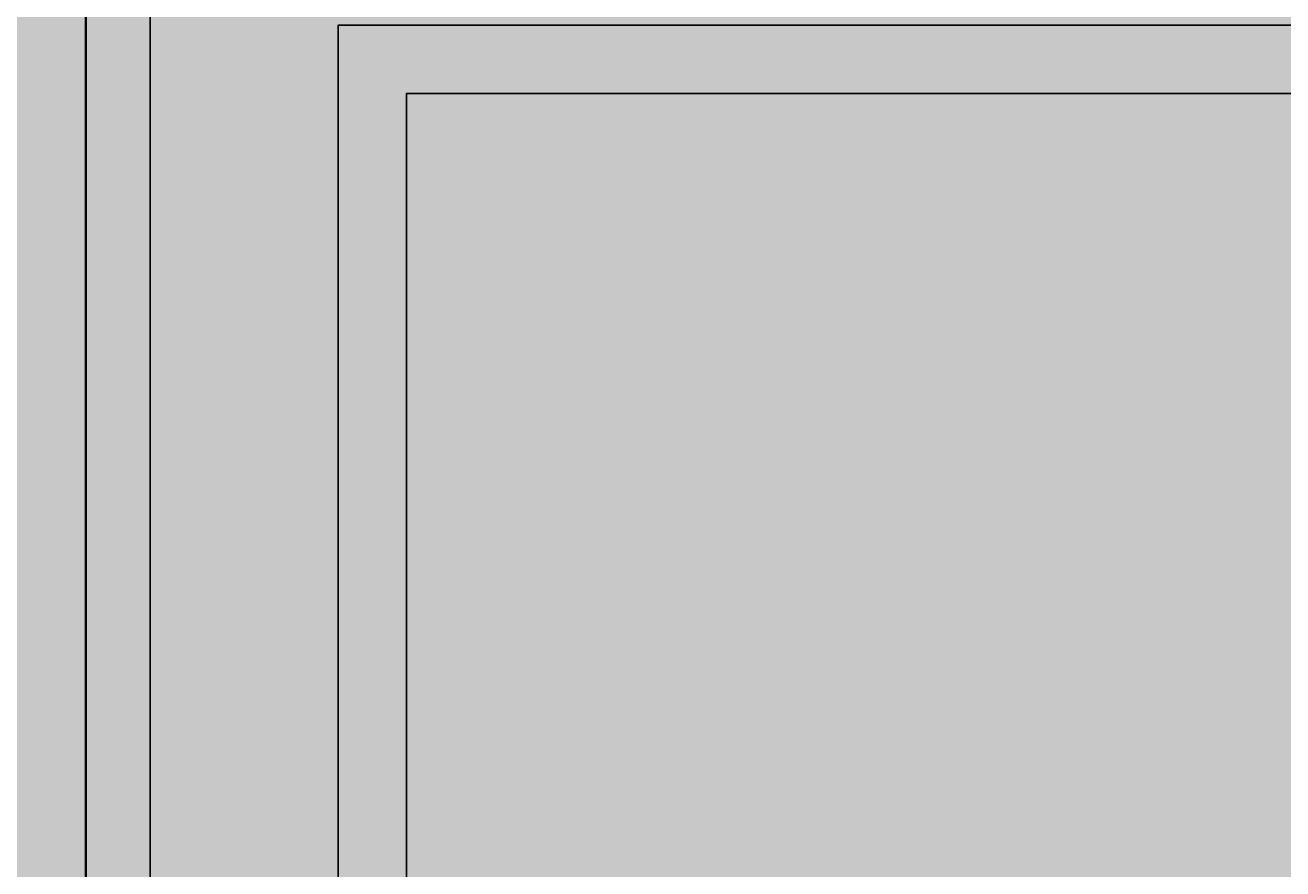
# Model space of a CAD drawing. Units: feet. Extents: x 2695 to 2912, y 795 to 1139.
# Tile 54 of 83: x 2769 to 2806, y 996 to 1021. Entities that reach past the tile are written whole.
import ezdxf

# ---------------------------------------------------------------- set-up
doc = ezdxf.new("R2010")
doc.units = ezdxf.units.FT
for name, color, linetype, lineweight in [('A-ANNO-DIMS', 2, 'Continuous', 18), ('A-ELEV', 7, 'Continuous', 35), ('A-ELEV-PATT', 252, 'Continuous', 13), ('A-GLAZ', 4, 'Continuous', 25), ('A-GLAZ-PATT', 254, 'Continuous', 13)]:
    doc.layers.add(name, color=color, linetype=linetype, lineweight=lineweight)
doc.styles.get("Standard").update_dxf_attribs({"font": 'arial.ttf'})
doc.dimstyles.get("Standard").update_dxf_attribs({"dimtxt": 0.18, "dimasz": 0.18, "dimexe": 0.18, "dimexo": 0.0625, "dimgap": 0.09, "dimtad": 0, "dimtih": 1, "dimtoh": 1, "dimdec": 1, "dimzin": 0, "dimdsep": 46, "dimlunit": 3, "dimtxsty": 'Standard', "dimcen": 0.09, "dimadec": 0, "dimazin": 0, "dimtfac": 1, "dimtdec": 1, "dimtofl": 0, "dimtmove": 0, "dimatfit": 3, "dimfxl": 1, "dimtolj": 1, "dimtzin": 0, "dimarcsym": 0})

# ---------------------------------------------------------------- blocks, each defined once
blk = doc.blocks.new('*D48')
at = {"layer": 'A-ANNO-DIMS', "color": 0, "lineweight": -2, "transparency": 16777216}
for p, q in [((2770.636, 972.03), (2770.636, 1138.886)), ((2770.816, 1138.706), (2771.263, 1138.706)), ((2772.342, 1138.706), (2771.894, 1138.706)), ((2772.522, 972.03), (2772.522, 1138.886))]:
    blk.add_line(p, q, dxfattribs=at)
at = {"layer": 'A-ANNO-DIMS', "color": 0, "transparency": 16777216}
for points in [[(2770.816, 1138.736), (2770.816, 1138.676), (2770.636, 1138.706)], [(2772.342, 1138.736), (2772.342, 1138.676), (2772.522, 1138.706)]]:
    blk.add_solid(points, dxfattribs=at)
at = {"layer": 'Defpoints', "color": 0, "transparency": 16777216}
for p in [(2772.522, 1138.706), (2770.636, 971.967), (2772.522, 971.967)]:
    blk.add_point(p, dxfattribs=at)
at = {"layer": 'A-ANNO-DIMS', "color": 0, "transparency": 16777216, "insert": (2771.579, 1138.706), "char_height": 0.18, "attachment_point": 5}
blk.add_mtext('\\A1;1.89', dxfattribs=at)
blk = doc.blocks.new('*D49')
at = {"layer": 'A-ANNO-DIMS', "color": 0, "lineweight": -2, "transparency": 16777216}
for p, q in [((2772.522, 972.03), (2772.522, 1138.886)), ((2772.702, 1138.706), (2790.888, 1138.706)), ((2809.861, 1138.706), (2791.674, 1138.706)), ((2810.041, 972.03), (2810.041, 1138.886))]:
    blk.add_line(p, q, dxfattribs=at)
at = {"layer": 'A-ANNO-DIMS', "color": 0, "transparency": 16777216}
for points in [[(2772.702, 1138.736), (2772.702, 1138.676), (2772.522, 1138.706)], [(2809.861, 1138.736), (2809.861, 1138.676), (2810.041, 1138.706)]]:
    blk.add_solid(points, dxfattribs=at)
at = {"layer": 'Defpoints', "color": 0, "transparency": 16777216}
for p in [(2810.041, 1138.706), (2772.522, 971.967), (2810.041, 971.967)]:
    blk.add_point(p, dxfattribs=at)
at = {"layer": 'A-ANNO-DIMS', "color": 0, "transparency": 16777216, "insert": (2791.281, 1138.706), "char_height": 0.18, "attachment_point": 5}
blk.add_mtext('\\A1;37.52', dxfattribs=at)

msp = doc.modelspace()

# ---------------------------------------------------------------- hatches: boundary and pattern name
at = {"layer": 'A-ELEV-PATT'}
h = msp.add_hatch(color=256, dxfattribs=at)
h.set_gradient(color1=(147, 149, 152), color2=(147, 149, 152), tint=1)
h.paths.add_polyline_path([(2770.6361, 1118.4096), (2710.6361, 1118.4096), (2710.6361, 1062.9306), (2770.6361, 1062.9306)])
h.paths.add_polyline_path([(2890.6361, 1103.3378), (2770.6361, 1103.3378), (2770.6361, 1062.9306), (2890.6361, 1062.9306)])
h.paths.add_polyline_path([(2730.7081, 1048.1052), (2755.1125, 1048.1052), (2755.1125, 936.9306), (2770.6361, 936.9306), (2770.6361, 1050.3105), (2715.8852, 1050.3105), (2715.8852, 936.9306), (2730.7081, 936.9306)])
h.paths.add_polyline_path([(2890.6361, 1050.3105), (2770.6361, 1050.3105), (2770.6361, 971.9673), (2778.0341, 971.9673), (2778.0341, 1020.8235), (2843.575, 1020.8235), (2843.575, 971.9673), (2890.6361, 971.9673)])
h.paths.add_polyline_path([(2888.1882, 970.7156), (2843.575, 970.7156), (2843.575, 964.8267), (2888.1882, 964.8267)])
h.paths.add_polyline_path([(2888.1882, 964.1328), (2843.575, 964.1328), (2843.575, 956.614), (2888.1882, 956.614)])
h.paths.add_polyline_path([(2888.1882, 955.9202), (2843.575, 955.9202), (2843.575, 949.2892), (2888.1882, 949.2892)])
h.paths.add_polyline_path([(2888.1882, 948.5954), (2843.575, 948.5954), (2843.575, 941.3507), (2888.1882, 941.3507)])
h.paths.add_polyline_path([(2888.1882, 940.6569), (2843.575, 940.6569), (2843.575, 936.9306), (2888.1882, 936.9306)])
h.paths.add_polyline_path([(2890.6361, 970.7156), (2888.9368, 970.7156), (2888.9368, 964.8267), (2890.6361, 964.8267)])
h.paths.add_polyline_path([(2890.6361, 964.1328), (2888.9368, 964.1328), (2888.9368, 956.614), (2890.6361, 956.614)])
h.paths.add_polyline_path([(2890.6361, 955.9202), (2888.9368, 955.9202), (2888.9368, 949.2892), (2890.6361, 949.2892)])
h.paths.add_polyline_path([(2890.6361, 940.6569), (2888.9368, 940.6569), (2888.9368, 936.9306), (2890.6361, 936.9306)])
h.paths.add_polyline_path([(2890.6361, 948.5954), (2888.9368, 948.5954), (2888.9368, 941.3507), (2890.6361, 941.3507)])
h.paths.add_polyline_path([(2772.5216, 970.7156), (2770.6361, 970.7156), (2770.6361, 964.8267), (2772.5216, 964.8267)])
h.paths.add_polyline_path([(2772.5216, 964.1328), (2770.6361, 964.1328), (2770.6361, 956.614), (2772.5216, 956.614)])
h.paths.add_polyline_path([(2772.5216, 955.9202), (2770.6361, 955.9202), (2770.6361, 949.2892), (2772.5216, 949.2892)])
h.paths.add_polyline_path([(2772.5216, 948.5954), (2770.6361, 948.5954), (2770.6361, 941.3507), (2772.5216, 941.3507)])
h.paths.add_polyline_path([(2772.5216, 940.6569), (2770.6361, 940.6569), (2770.6361, 936.9306), (2772.5216, 936.9306)])
h.paths.add_polyline_path([(2778.0341, 940.6569), (2773.2702, 940.6569), (2773.2702, 936.9306), (2778.0341, 936.9306)])
h.paths.add_polyline_path([(2778.0341, 970.7156), (2773.2702, 970.7156), (2773.2702, 964.8267), (2778.0341, 964.8267)])
h.paths.add_polyline_path([(2778.0341, 964.1328), (2773.2702, 964.1328), (2773.2702, 956.614), (2778.0341, 956.614)])
h.paths.add_polyline_path([(2778.0341, 955.9202), (2773.2702, 955.9202), (2773.2702, 949.2892), (2778.0341, 949.2892)])
h.paths.add_polyline_path([(2778.0341, 948.5954), (2773.2702, 948.5954), (2773.2702, 941.3507), (2778.0341, 941.3507)])
h.paths.add_polyline_path([(2810.0407, 940.6569), (2780.0341, 940.6569), (2780.0341, 936.9306), (2810.0407, 936.9306)])
h.paths.add_polyline_path([(2890.6361, 924.3105), (2770.6361, 924.3105), (2770.6361, 810.9306), (2773.5029, 810.9306), (2773.5029, 905.5143), (2805.9398, 905.5143), (2838.3767, 905.5143), (2838.3767, 810.9306), (2890.6361, 810.9306)])
h = msp.add_hatch(color=256, dxfattribs=at)
h.set_gradient(color2=(0, 0, 0), tint=1)
h.paths.add_polyline_path([(2772.5216, 971.9673), (2770.6361, 971.9673), (2770.6361, 970.7156), (2772.5216, 970.7156)])
h.paths.add_polyline_path([(2773.2702, 971.9673), (2772.5216, 971.9673), (2772.5216, 970.7156), (2773.2702, 970.7156)])
h.paths.add_polyline_path([(2778.0341, 971.9673), (2773.2702, 971.9673), (2773.2702, 970.7156), (2778.0341, 970.7156)])
h.paths.add_polyline_path([(2780.0341, 971.9673), (2778.0341, 971.9673), (2778.0341, 970.7156), (2780.0341, 970.7156)])
h.paths.add_polyline_path([(2841.575, 971.9673), (2780.0341, 971.9673), (2780.0341, 970.7156), (2841.575, 970.7156)])
h.paths.add_polyline_path([(2843.575, 971.9673), (2841.575, 971.9673), (2841.575, 970.7156), (2843.575, 970.7156)])
h.paths.add_polyline_path([(2888.1882, 971.9673), (2843.575, 971.9673), (2843.575, 970.7156), (2888.1882, 970.7156)])
h.paths.add_polyline_path([(2888.9368, 971.9673), (2888.1882, 971.9673), (2888.1882, 970.7156), (2888.9368, 970.7156)], flags=17)
h.paths.add_polyline_path([(2890.6361, 971.9673), (2888.9368, 971.9673), (2888.9368, 970.7156), (2890.6361, 970.7156)])
h.paths.add_polyline_path([(2888.9368, 971.9673), (2888.1882, 971.9673), (2888.1882, 964.8267), (2888.9368, 964.8267)])
h.paths.add_polyline_path([(2888.9368, 964.8267), (2888.1882, 964.8267), (2888.1882, 964.1328), (2888.9368, 964.1328)])
h.paths.add_polyline_path([(2890.6361, 964.8267), (2888.9368, 964.8267), (2888.9368, 964.1328), (2890.6361, 964.1328)])
h.paths.add_polyline_path([(2888.1882, 964.8267), (2770.6361, 964.8267), (2770.6361, 964.1328), (2888.1882, 964.1328)])
h.paths.add_polyline_path([(2888.9368, 964.1328), (2888.1882, 964.1328), (2888.1882, 936.9306), (2888.9368, 936.9306)])
h.paths.add_polyline_path([(2890.6361, 956.614), (2888.9368, 956.614), (2888.9368, 955.9202), (2890.6361, 955.9202)])
h.paths.add_polyline_path([(2888.1882, 956.614), (2770.6361, 956.614), (2770.6361, 955.9202), (2888.1882, 955.9202)])
h.paths.add_polyline_path([(2890.6361, 949.2892), (2888.9368, 949.2892), (2888.9368, 948.5954), (2890.6361, 948.5954)])
h.paths.add_polyline_path([(2888.1882, 949.2892), (2770.6361, 949.2892), (2770.6361, 948.5954), (2888.1882, 948.5954)])
h.paths.add_polyline_path([(2890.6361, 941.3507), (2888.9368, 941.3507), (2888.9368, 940.6569), (2890.6361, 940.6569)])
h.paths.add_polyline_path([(2888.1882, 941.3507), (2770.6361, 941.3507), (2770.6361, 940.6569), (2888.1882, 940.6569)])
h.paths.add_polyline_path([(2773.2702, 970.7156), (2772.5216, 970.7156), (2772.5216, 964.8267), (2773.2702, 964.8267)])
h.paths.add_polyline_path([(2773.2702, 964.1328), (2772.5216, 964.1328), (2772.5216, 956.614), (2773.2702, 956.614)])
h.paths.add_polyline_path([(2773.2702, 955.9202), (2772.5216, 955.9202), (2772.5216, 936.9306), (2773.2702, 936.9306)])
h.paths.add_polyline_path([(2810.7893, 970.7156), (2810.0407, 970.7156), (2810.0407, 964.8267), (2810.7893, 964.8267)], flags=17)
h.paths.add_polyline_path([(2810.7893, 964.1328), (2810.0407, 964.1328), (2810.0407, 956.614), (2810.7893, 956.614)], flags=17)
h.paths.add_polyline_path([(2810.7893, 955.9202), (2810.0407, 955.9202), (2810.0407, 949.2892), (2810.7893, 949.2892)], flags=17)
h.paths.add_polyline_path([(2810.7893, 971.9673), (2810.0407, 971.9673), (2810.0407, 941.3507), (2810.7893, 941.3507)])
h.paths.add_polyline_path([(2810.7893, 940.6569), (2810.0407, 940.6569), (2810.0407, 936.9306), (2810.7893, 936.9306)])
h.paths.add_polyline_path([(2780.0341, 1018.8235), (2841.575, 1018.8235), (2841.575, 971.9673), (2843.575, 971.9673), (2843.575, 1020.8235), (2778.0341, 1020.8235), (2778.0341, 971.9673), (2780.0341, 971.9673)])
h.paths.add_polyline_path([(2780.0341, 970.7156), (2778.0341, 970.7156), (2778.0341, 964.8267), (2780.0341, 964.8267)])
h.paths.add_polyline_path([(2780.0341, 964.1328), (2778.0341, 964.1328), (2778.0341, 956.614), (2780.0341, 956.614)])
h.paths.add_polyline_path([(2780.0341, 955.9202), (2778.0341, 955.9202), (2778.0341, 949.2892), (2780.0341, 949.2892)])
h.paths.add_polyline_path([(2780.0341, 948.5954), (2778.0341, 948.5954), (2778.0341, 941.3507), (2780.0341, 941.3507)])
h.paths.add_polyline_path([(2780.0341, 940.6569), (2778.0341, 940.6569), (2778.0341, 936.9306), (2780.0341, 936.9306)])
h.paths.add_polyline_path([(2843.575, 940.6569), (2841.575, 940.6569), (2841.575, 936.9306), (2843.575, 936.9306)])
h.paths.add_polyline_path([(2843.575, 948.5954), (2841.575, 948.5954), (2841.575, 941.3507), (2843.575, 941.3507)])
h.paths.add_polyline_path([(2843.575, 970.7156), (2841.575, 970.7156), (2841.575, 964.8267), (2843.575, 964.8267)])
h.paths.add_polyline_path([(2843.575, 964.1328), (2841.575, 964.1328), (2841.575, 956.614), (2843.575, 956.614)])
h.paths.add_polyline_path([(2843.575, 955.9202), (2841.575, 955.9202), (2841.575, 949.2892), (2843.575, 949.2892)])
h.paths.add_polyline_path([(2805.0538, 874.1057), (2803.9681, 874.1057), (2803.9681, 846.2857), (2805.0538, 846.2857)])
h.paths.add_polyline_path([(2758.1515, 902.577), (2724.1893, 902.577), (2724.1893, 874.8571), (2758.1515, 874.8571)])
h.paths.add_polyline_path([(2726.1893, 900.577), (2756.1515, 900.577), (2756.1515, 876.8571), (2726.1893, 876.8571)], flags=16)
h.paths.add_polyline_path([(2740.7302, 900.577), (2741.6105, 900.577), (2741.6105, 876.8571), (2740.7302, 876.8571)], flags=0)
at = {"layer": 'A-GLAZ-PATT'}
h = msp.add_hatch(color=256, dxfattribs=at)
h.set_gradient(color1=(213, 227, 240), color2=(213, 227, 240))
h.paths.add_polyline_path([(2810.8045, 1018.8235), (2780.0341, 1018.8235), (2780.0341, 971.9673), (2810.8045, 971.9673)])
h.paths.add_polyline_path([(2841.575, 1018.8235), (2810.8045, 1018.8235), (2810.8045, 971.9673), (2841.575, 971.9673)])
h.paths.add_polyline_path([(2810.0407, 970.7156), (2780.0341, 970.7156), (2780.0341, 964.8267), (2810.0407, 964.8267)])
h.paths.add_polyline_path([(2841.575, 970.7156), (2810.8045, 970.7156), (2810.8045, 964.8267), (2841.575, 964.8267)])
h.paths.add_polyline_path([(2841.575, 964.1328), (2810.8045, 964.1328), (2810.8045, 956.614), (2841.575, 956.614)])
h.paths.add_polyline_path([(2810.0407, 964.1328), (2780.0341, 964.1328), (2780.0341, 956.614), (2810.0407, 956.614)])
h.paths.add_polyline_path([(2810.0407, 955.9202), (2780.0341, 955.9202), (2780.0341, 949.2892), (2810.0407, 949.2892)])
h.paths.add_polyline_path([(2841.575, 955.9202), (2810.8045, 955.9202), (2810.8045, 949.2892), (2841.575, 949.2892)])
h.paths.add_polyline_path([(2841.575, 948.5954), (2810.8045, 948.5954), (2810.8045, 941.3507), (2841.575, 941.3507)])
h.paths.add_polyline_path([(2810.0407, 948.5954), (2780.0341, 948.5954), (2780.0341, 941.3507), (2810.0407, 941.3507)])
h.paths.add_polyline_path([(2810.0407, 940.6569), (2780.0341, 940.6569), (2780.0341, 936.9306), (2810.0407, 936.9306)])
h.paths.add_polyline_path([(2841.575, 940.6569), (2810.8045, 940.6569), (2810.8045, 936.9306), (2841.575, 936.9306)])

# ---------------------------------------------------------------- linework, layer by layer
at = {"layer": 'A-ELEV'}
msp.add_line((2770.6361, 1050.3105), (2770.6361, 936.9306), dxfattribs=at)
at = {"layer": 'A-GLAZ'}
for points in [[(2778.0341, 936.9306), (2778.0341, 1020.8235), (2843.575, 1020.8235), (2843.575, 936.9306)], [(2780.0341, 936.9306), (2780.0341, 1018.8235), (2841.575, 1018.8235), (2841.575, 936.9306)]]:
    msp.add_lwpolyline(points, dxfattribs=at)

# ---------------------------------------------------------------- dimensions: what is measured, and where the dimension line sits
at = {"layer": 'A-ANNO-DIMS'}
for base, p1, p2, picture, middle in [((2772.5216, 1138.7056), (2770.6361, 971.9673), (2772.5216, 971.9673), '*D48', (2771.5788, 1138.7056)), ((2810.0407, 1138.7056), (2772.5216, 971.9673), (2810.0407, 971.9673), '*D49', (2791.2811, 1138.7056))]:
    dim = msp.add_linear_dim(base=base, p1=p1, p2=p2, dimstyle='Standard', override={"dimdec": 2, "dimlfac": 1, "dimrnd": 0, "dimzin": 0, "dimdsep": 46, "dimlunit": 2}, dxfattribs=at)
    dim.commit()
    dim.dimension.update_dxf_attribs({"geometry": picture, "text_midpoint": middle})

doc.saveas('drawing.dxf')
